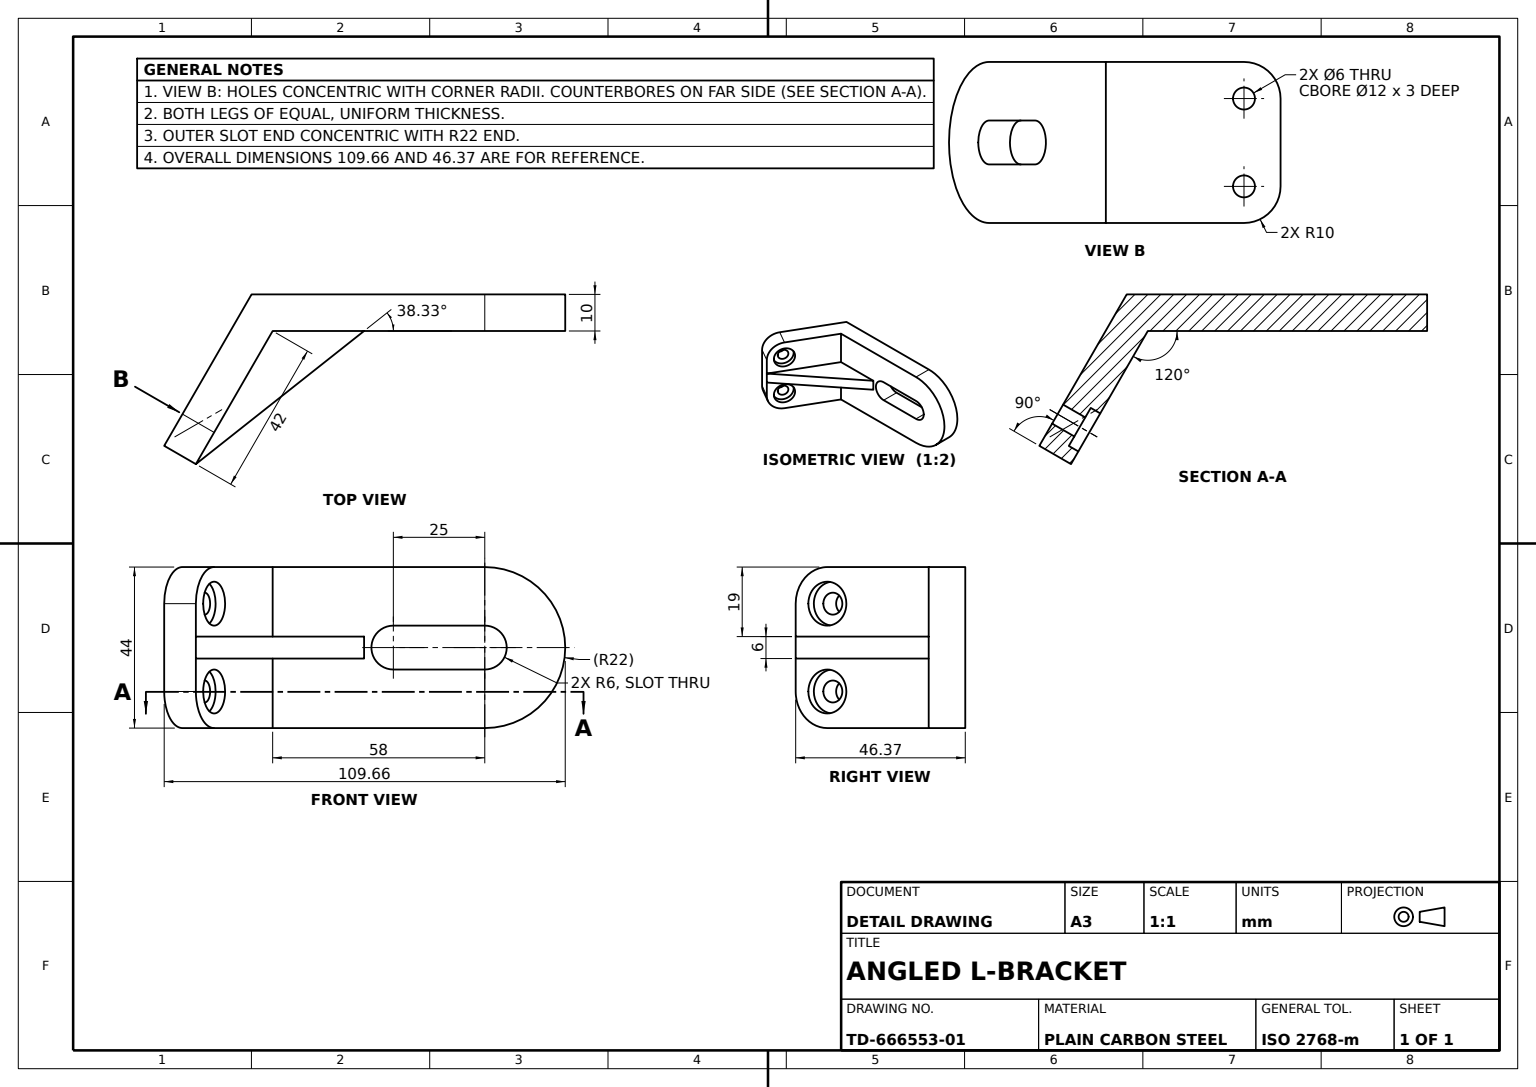
SolidWorks part; units mm, degrees
material "Plain Carbon Steel"
ref_plane "Front Plane" through (0, 0, 0) normal (0, 0, 1) x (1, 0, 0)
ref_plane "Top Plane" through (0, 0, 0) normal (0, 1, 0) x (1, 0, 0)
ref_plane "Right Plane" through (0, 0, 0) normal (1, 0, 0) x (0, 0, -1)
sketch "Base Plate Sketch" plane through (0, 0, 0) normal (0, 0, 1) x (1, 0, 0)
  line L0 (0, 0) -> (58, 0)
  line L1 (0, 0) -> (0, 44)
  line L2 (0, 44) -> (58, 44)
  line L3 (58, 44) -> (58, 0)
  dimension "D1" = 58
  dimension "D2" = 44
extrude "Base Plate 58x44x10" add sketch "Base Plate Sketch" along normal blind 10
sketch "Base Rounded End Sketch" plane through (0, 0, 10) normal (0, 0, 1) x (1, 0, 0)
  line L0 (58, 0) -> (58, 44) construction
  circle A0 centre (58, 22) radius 22
  dimension "D1" = 22
extrude "Base Rounded End R22" add sketch "Base Rounded End Sketch" against normal blind 10
sketch "Base Slot Sketch" plane through (0, 0, 10) normal (0, 0, 1) x (1, 0, 0)
  line L1 (33, 28) -> (58, 28)
  line L2 (33, 16) -> (58, 16)
  arc A0 (58, 16) -> (58, 28) centre (58, 22) ccw
  arc A1 (33, 28) -> (33, 16) centre (33, 22) ccw
  dimension "D1" = 6
  dimension "D3" = 6
  dimension "D4" = 25
  dimension "D5" = 25
extrude "Base Slot" cut sketch "Base Slot Sketch" against normal blind 10
sketch "Angled Arm Sketch" plane through (0, 0, 0) normal (0, -1, 0) x (1, 0, 0)
  line L0 (0, 10) -> (-21, 46.3731)
  line L1 (0, 10) -> (58, 10) construction
  line L2 (0, 10) -> (-21, 46.3731)
  line L3 (-21, 46.3731) -> (-29.6603, 41.3731)
  line L4 (-29.6603, 41.3731) -> (-5.7735, 0)
  line L5 (-5.7735, 0) -> (0, 0)
  line L6 (0, 0) -> (5.7735, 0)
  line L7 (0, 0) -> (58, 0) construction
  line L8 (5.7735, 0) -> (0, 10)
  line M5 (0, 10) -> (0, 0)
  dimension "D1" = 120
  dimension "D2" = 42
  dimension "D3" = 10
extrude "Angled Arm 120deg" add sketch "Angled Arm Sketch" against normal blind 44 contours L4 L5 L0 L3 M5
sketch "Arm End Trim Sketch" plane through (4.3301, 0, 2.5) normal (0.866, 0, 0.5) x (0.5, 0, -0.866)
  line L0 (-50.6603, 0) -> (-40.6603, 0)
  line L1 (-8.6603, 0) -> (-50.6603, 0) construction
  line L3 (-50.6603, 44) -> (-40.6603, 44)
  line L4 (-8.6603, 44) -> (-50.6603, 44) construction
  line L8 (-50.6603, 0) -> (-50.6603, 10)
  line L9 (-50.6603, 44) -> (-50.6603, 34)
  arc A0 (-50.6603, 10) -> (-40.6603, 0) centre (-40.6603, 10) ccw
  arc A1 (-40.6603, 44) -> (-50.6603, 34) centre (-40.6603, 34) ccw
  dimension "D1" = 10
  dimension "D2" = 10
  dimension "D4" = 10
  dimension "D5" = 10
extrude "Arm End Trim" cut sketch "Arm End Trim Sketch" against normal blind 10
sketch "Counterbore Sketch" plane through (4.3301, 0, 2.5) normal (0.866, 0, 0.5) x (0.5, 0, -0.866)
  circle A0 centre (-40.6603, 34) radius 6
  circle A1 centre (-40.6603, 10) radius 6
  dimension "D1" = 12
  dimension "D2" = 12
extrude "Counterbores 2xØ12x3" cut sketch "Counterbore Sketch" against normal blind 3
sketch "Arm Hole Sketch" plane through (1.7321, 0, 1) normal (0.866, 0, 0.5) x (0.5, 0, -0.866)
  circle A0 centre (-40.6603, 34) radius 3
  circle A1 centre (-40.6603, 10) radius 3
  dimension "D1" = 6
  dimension "D2" = 6
extrude "Arm Holes 2xØ6" cut sketch "Arm Hole Sketch" against normal blind 10
sketch "Gusset Profile Sketch" plane through (0, 0, 0) normal (0, -1, 0) x (1, 0, 0)
  line L0 (0, 10) -> (25, 10)
  line L1 (0, 10) -> (58, 10) construction
  line L2 (25, 10) -> (-21, 46.3731)
  line L3 (-21, 46.3731) -> (0, 10)
  dimension "D1" = 25
extrude "Gusset Blank" add sketch "Gusset Profile Sketch" against normal blind 44
sketch "Gusset Side Trim 1 Sketch" plane through (0, 0, 0) normal (0, -1, 0) x (1, 0, 0)
  line L1 (4.8916, 10) -> (25, 10)
  line L2 (25, 10) -> (-21, 46.3731)
  line L3 (-21, 46.3731) -> (0, 10)
  line L4 (0, 10) -> (4.8916, 10)
  dimension "D1" = 53.1084
  dimension "D2" = 58
extrude "Gusset Side Trim 1" cut sketch "Gusset Side Trim 1 Sketch" against normal blind 19
sketch "Gusset Side Trim 2 Sketch" plane through (0, 44, 0) normal (0, 1, 0) x (1, 0, 0)
  line L0 (25, -10) -> (0, -10)
  line L1 (0, -10) -> (-21, -46.3731)
  line L2 (-21, -46.3731) -> (25, -10)
  dimension "D1" = 25
extrude "Gusset Side Trim 2" cut sketch "Gusset Side Trim 2 Sketch" against normal blind 19
